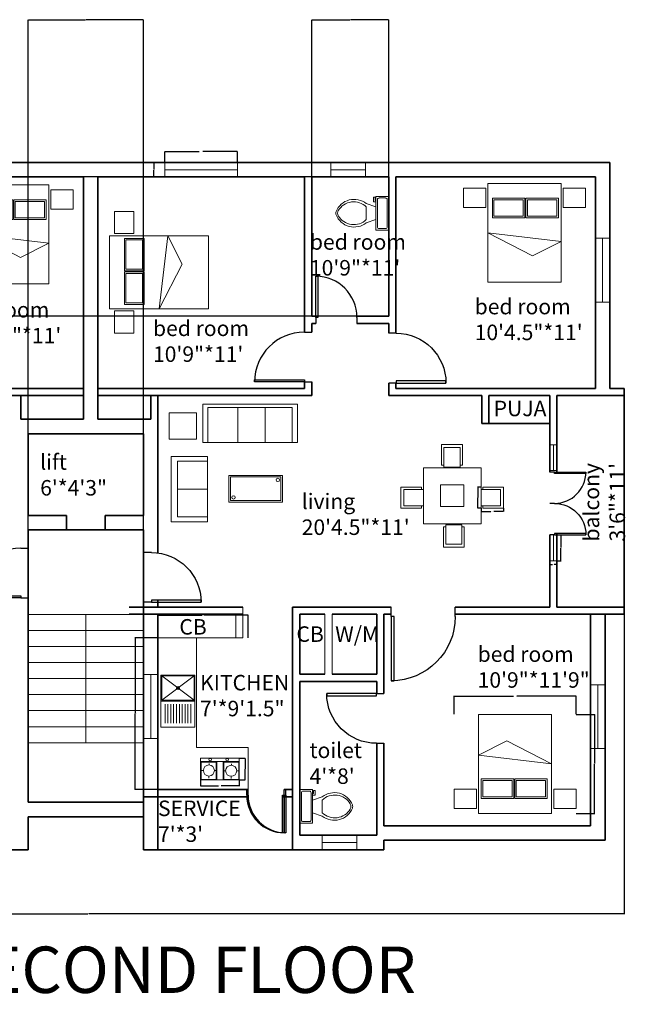
# Model space of a CAD drawing. Units: inches. Extents: x 1632 to 2336, y 1480 to 2095.
# Tile 2 of 2: x 1958 to 2336, y 1480 to 2095. Entities that reach past the tile are written whole.
import ezdxf

# ---------------------------------------------------------------- set-up
doc = ezdxf.new("R2010")
doc.units = ezdxf.units.IN
for name, color, linetype, lineweight in [('A-ANNO-DIMS', 2, 'Continuous', 18), ('A-ANNO-TEXT', 7, 'Continuous', 18), ('A-ANNO-TITL', 7, 'Continuous', 35), ('A-AREA-IDEN', 7, 'Continuous', 18), ('A-DOOR', 3, 'Continuous', 25), ('A-EQPM', 8, 'Continuous', 18), ('A-FLOR-CASE', 9, 'Continuous', 18), ('A-FLOR-FIXT', 9, 'Continuous', 18), ('A-FLOR-STRS', 7, 'Continuous', 18), ('A-FURN', 8, 'Continuous', 18), ('A-GLAZ', 4, 'Continuous', 18), ('A-WALL', 7, 'Continuous', 35)]:
    doc.layers.add(name, color=color, linetype=linetype, lineweight=lineweight)
doc.styles.get("Standard").update_dxf_attribs({"font": 'arial.ttf'})
doc.dimstyles.get("Standard").update_dxf_attribs({"dimtxt": 0.18, "dimasz": 0.18, "dimexe": 0.18, "dimexo": 0.0625, "dimgap": 0.09, "dimtad": 0, "dimtih": 1, "dimtoh": 1, "dimdec": 4, "dimzin": 0, "dimdsep": 46, "dimtxsty": 'Standard', "dimcen": 0.09, "dimadec": 0, "dimazin": 0, "dimtfac": 1, "dimtdec": 4, "dimtofl": 0, "dimtmove": 0, "dimatfit": 3, "dimfxl": 1, "dimtolj": 1, "dimtzin": 0, "dimarcsym": 0})

# ---------------------------------------------------------------- blocks, each defined once
blk = doc.blocks.new('*U2')
for p, q in [((0, 0), (0, -6)), ((40, 0), (40, -6))]:
    blk.add_line(p, q)
blk.add_lwpolyline([(0, 0), (0, 40), (1.75, 40), (1.75, 0)], close=True)
blk.add_arc((0, 0), 40, 0, 90)
blk = doc.blocks.new('*U4')
for p, q in [((9.5, -6), (9.5, -2)), ((-10, -8.5), (-8, -8.5)), ((-10, -9.5), (-10, -8.5)), ((-7, -9.5), (-10, -9.5)), ((-8, -8.5), (-8, -8)), ((-7, -8), (-7, -9.5)), ((-4, -8), (-6, -14)), ((4, -8), (6, -14)), ((4, -14), (-4, -14))]:
    blk.add_line(p, q)
blk.add_lwpolyline([(10.5, -8), (10.5, 0), (-10.5, 0), (-10.5, -8)], close=True)
for points in [[(-9.5, -2), (-9.5, -6)], [(8.5, -1), (-8.5, -1)], [(-8.5, -7), (8.5, -7)]]:
    blk.add_lwpolyline(points)
for centre, radius, start, end in [((-8.62, -1.88), 0.884, 81.8699, 188.1301), ((-8.62, -6.12), 0.884, 171.8699, 278.1301), ((8.62, -1.88), 0.884, 351.8699, 98.1301), ((8.62, -6.12), 0.884, 261.8699, 8.1301), ((3.52, -21.58), 12.17, 141.46911, 247.97143), ((4.2, -21.82), 11.33, 136.36773, 238.94682), ((-3.52, -21.58), 12.17, 292.02843, 38.53071), ((-4.2, -21.82), 11.33, 301.05301, 43.63209), ((0, -27.88), 4, 245.73182, 294.26817), ((0, -29), 4, 254.86053, 285.13947)]:
    blk.add_arc(centre, radius, start, end)
blk = doc.blocks.new('BED-DOUBLE-WITH-NIGHTSTANDS')
for p, q in [((30.9, 15.3), (36.28, 60.91)), ((36.28, 60.91), (45.27, 43.14)), ((45.27, 43.14), (30.9, 15.3))]:
    blk.add_line(p, q)
for points in [[(3.09, 62.18), (15.1, 62.18), (15.1, 76.08), (3.09, 76.08)], [(0, 15.3), (61.8, 15.3), (61.8, 60.91), (0, 60.91)], [(9.26, 38.94), (21.51, 38.94), (21.51, 59.23), (9.26, 59.23)], [(10.26, 39.94), (20.51, 39.94), (20.51, 58.23), (10.26, 58.23)], [(9.26, 18.02), (21.51, 18.02), (21.51, 38.31), (9.26, 38.31)], [(10.26, 19.02), (20.51, 19.02), (20.51, 37.31), (10.26, 37.31)], [(3.09, 0), (15.1, 0), (15.1, 13.9), (3.09, 13.9)]]:
    blk.add_lwpolyline(points, close=True)
blk = doc.blocks.new('CHAIR-DINING')
for p, q in [((0, 1.12), (0, 13.97)), ((0, 13.97), (12.95, 13.97)), ((12.95, 13.97), (12.95, 1.12)), ((1.47, 1.12), (0, 1.12)), ((12.95, 1.12), (11.55, 1.12))]:
    blk.add_line(p, q)
blk.add_lwpolyline([(1.47, 0), (11.55, 0), (11.55, 12.08), (1.47, 12.08)], close=True)
blk = doc.blocks.new('TABLE-DINING')
for points in [[(0, 35.03), (36, 35.03), (36, 0), (0, 0)], [(10.77, 24.25), (25.23, 24.25), (25.23, 10.77), (10.77, 10.77)]]:
    blk.add_lwpolyline(points, close=True)
blk = doc.blocks.new('SOFA-3-SEAT')
for p, q in [((0, 0), (0, 24.07)), ((0, 24.07), (59, 24.07)), ((20.13, 21.83), (20.13, 0)), ((37.25, 21.83), (37.25, 0)), ((59, 0), (59, 24.07)), ((3.41, 0), (0, 0)), ((56, 0), (59, 0))]:
    blk.add_line(p, q)
blk.add_lwpolyline([(3.41, 21.83), (56, 21.83), (56, 0), (3.41, 0)], close=True)
blk = doc.blocks.new('SOFA-2-SEAT')
for p, q in [((0, 37.84), (0, 40.84)), ((0, 40.84), (22.7, 40.84)), ((22.7, 40.84), (22.7, 0)), ((0, 20.42), (18.79, 20.42)), ((0, 3), (0, 0)), ((0, 0), (22.7, 0))]:
    blk.add_line(p, q)
blk.add_lwpolyline([(18.79, 37.84), (0, 37.84), (0, 3), (18.79, 3)], close=True)
blk = doc.blocks.new('TABLE-COFFEE')
for points in [[(0, 16.65), (33.49, 16.65), (33.49, 0), (0, 0)], [(1, 15.65), (32.49, 15.65), (32.49, 1), (1, 1)]]:
    blk.add_lwpolyline(points, close=True)
for centre in [(2.89, 13.8), (30.54, 2.86)]:
    blk.add_circle(centre, 1.06)
blk = doc.blocks.new('SINK-WITH-DRAINBOARD')
for p, q in [((0.63, 16.78), (20.68, 31.97)), ((0.63, 31.97), (20.68, 16.78)), ((0, 16.25), (21.16, 16.25)), ((2.61, 14.26), (2.61, 2.54)), ((4.39, 14.26), (4.39, 2.54)), ((6.16, 14.26), (6.16, 2.54)), ((7.94, 14.26), (7.94, 2.54)), ((9.72, 14.26), (9.72, 2.54)), ((11.49, 14.26), (11.49, 2.54)), ((13.27, 14.26), (13.27, 2.54)), ((15.04, 14.26), (15.04, 2.54)), ((16.82, 14.26), (16.82, 2.54)), ((18.6, 14.26), (18.6, 2.54))]:
    blk.add_line(p, q)
for points in [[(0, 0), (21.16, 0), (21.16, 32.49), (0, 32.49)], [(0.63, 31.97), (20.68, 31.97), (20.68, 16.78), (0.63, 16.78)]]:
    blk.add_lwpolyline(points, close=True)
blk.add_circle((10.66, 24.37), 0.977)
blk = doc.blocks.new('COOKTOP-2-BURNER')
for p, q in [((0, 11.46), (0, 13.65)), ((0, 13.65), (24.07, 13.65)), ((24.07, 13.65), (24.07, 11.46)), ((0, 11.46), (12, 11.46)), ((0, 11.46), (10, 11.46)), ((5.23, 9.36), (5.23, 10.33)), ((10, 11.46), (10, 0)), ((24.07, 11.46), (14.07, 11.46)), ((14.07, 11.46), (14.07, 0)), ((19.15, 9.18), (19.15, 10.15)), ((1.67, 5.97), (0.82, 5.97)), ((5.05, 2.47), (5.05, 1.13)), ((8.57, 5.88), (9.52, 5.88)), ((15.59, 5.79), (14.74, 5.79)), ((18.97, 2.28), (18.97, 0.95)), ((22.49, 5.7), (23.44, 5.7))]:
    blk.add_line(p, q)
for points in [[(0, 11.46), (24.07, 11.46), (24.07, 0), (0, 0)], [(0.38, 11.07), (9.77, 11.07), (9.77, 0.28), (0.38, 0.28)], [(14.37, 11.14), (23.83, 11.14), (23.83, 0.28), (14.37, 0.28)]]:
    blk.add_lwpolyline(points, close=True)
for centre, radius in [((5.93, 12.7), 0.782), ((16.53, 12.66), 0.782), ((5.12, 5.91), 3.45), ((19.04, 5.73), 3.45)]:
    blk.add_circle(centre, radius)
blk = doc.blocks.new('WINDOW-40')
blk.add_line((4.5, 39.93), (4.5, 0))
blk.add_lwpolyline([(0, 39.93), (9, 39.93), (9, 0), (0, 0)], close=True)
blk = doc.blocks.new('WINDOW-22')
blk.add_line((0, 4.5), (21.58, 4.5))
blk.add_lwpolyline([(0, 9), (21.58, 9), (21.58, 0), (0, 0)], close=True)
blk = doc.blocks.new('WINDOW-45')
blk.add_line((0, 4.5), (45.36, 4.5))
blk.add_lwpolyline([(0, 9), (45.36, 9), (45.36, 0), (0, 0)], close=True)
blk = doc.blocks.new('WINDOW-SIDELIGHT-16')
blk.add_line((2.25, 0), (2.25, 16.22))
blk.add_lwpolyline([(4.5, 0), (0, 0), (0, 16.22), (4.5, 16.22)], close=True)
blk = doc.blocks.new('TABLE-END')
blk.add_lwpolyline([(0, 16.51), (17.12, 16.51), (17.12, 0), (0, 0)], close=True)
blk = doc.blocks.new('COUNTERTOP-L-RETURN')
for p, q in [((0, 94.74), (24, 94.74)), ((24, 94.74), (24, 26.35)), ((24, 26.35), (56.24, 26.35)), ((56.24, 0), (56.24, 26.35))]:
    blk.add_line(p, q)
blk = doc.blocks.new('*D20')
at = {"layer": 'A-ANNO-DIMS', "color": 0, "lineweight": -2, "transparency": 16777216}
for p, q in [((2229, 1661.18), (2229, 1672.71)), ((2229.18, 1672.53), (2265.94, 1672.53)), ((2304.9, 1672.53), (2268.14, 1672.53)), ((2305.08, 1661.18), (2305.08, 1672.71))]:
    blk.add_line(p, q, dxfattribs=at)
at = {"layer": 'A-ANNO-DIMS', "color": 0, "transparency": 16777216}
for points in [[(2229.18, 1672.56), (2229.18, 1672.5), (2229, 1672.53)], [(2304.9, 1672.56), (2304.9, 1672.5), (2305.08, 1672.53)]]:
    blk.add_solid(points, dxfattribs=at)
at = {"layer": 'Defpoints', "color": 0, "transparency": 16777216}
for p in [(2229, 1672.53), (2229, 1661.12), (2305.08, 1661.12)]:
    blk.add_point(p, dxfattribs=at)
at = {"layer": 'A-ANNO-DIMS', "color": 0, "transparency": 16777216, "insert": (2267.04, 1672.53), "char_height": 0.18, "attachment_point": 5}
blk.add_mtext('\\A1;BED SET 76 TYP.', dxfattribs=at)
blk = doc.blocks.new('*D21')
at = {"layer": 'A-ANNO-DIMS', "color": 0, "lineweight": -2, "transparency": 16777216}
for p, q in [((2305.14, 1661.12), (2316.67, 1661.12)), ((2316.49, 1660.94), (2316.49, 1630.4)), ((2316.49, 1599.5), (2316.49, 1630.04)), ((2305.14, 1599.32), (2316.67, 1599.32))]:
    blk.add_line(p, q, dxfattribs=at)
at = {"layer": 'A-ANNO-DIMS', "color": 0, "transparency": 16777216}
for points in [[(2316.46, 1660.94), (2316.52, 1660.94), (2316.49, 1661.12)], [(2316.46, 1599.5), (2316.52, 1599.5), (2316.49, 1599.32)]]:
    blk.add_solid(points, dxfattribs=at)
at = {"layer": 'Defpoints', "color": 0, "transparency": 16777216}
for p in [(2305.08, 1661.12), (2316.49, 1661.12), (2305.08, 1599.32)]:
    blk.add_point(p, dxfattribs=at)
at = {"layer": 'A-ANNO-DIMS', "color": 0, "transparency": 16777216, "insert": (2316.49, 1630.22), "char_height": 0.18, "attachment_point": 5}
blk.add_mtext('\\A1;62 TYP.', dxfattribs=at)
blk = doc.blocks.new('*D22')
at = {"layer": 'A-ANNO-DIMS', "color": 0, "lineweight": -2, "transparency": 16777216}
for p, q in [((2245.75, 1789.88), (2245.75, 1787.66)), ((2259.72, 1789.88), (2259.72, 1787.66)), ((2245.93, 1787.84), (2251.78, 1787.84)), ((2259.54, 1787.84), (2253.69, 1787.84))]:
    blk.add_line(p, q, dxfattribs=at)
at = {"layer": 'A-ANNO-DIMS', "color": 0, "transparency": 16777216}
for points in [[(2245.93, 1787.87), (2245.93, 1787.81), (2245.75, 1787.84)], [(2259.54, 1787.87), (2259.54, 1787.81), (2259.72, 1787.84)]]:
    blk.add_solid(points, dxfattribs=at)
at = {"layer": 'Defpoints', "color": 0, "transparency": 16777216}
for p in [(2245.75, 1789.94), (2259.72, 1789.94), (2259.72, 1787.84)]:
    blk.add_point(p, dxfattribs=at)
at = {"layer": 'A-ANNO-DIMS', "color": 0, "transparency": 16777216, "insert": (2252.74, 1787.84), "char_height": 0.18, "attachment_point": 5}
blk.add_mtext('\\A1;CHAIR 14 TYP.', dxfattribs=at)
blk = doc.blocks.new('*D23')
at = {"layer": 'A-ANNO-DIMS', "color": 0, "lineweight": -2, "transparency": 16777216}
for p, q in [((2245.69, 1802.89), (2243.48, 1802.89)), ((2243.66, 1802.71), (2243.66, 1796.6)), ((2243.66, 1790.12), (2243.66, 1796.23)), ((2245.69, 1789.94), (2243.48, 1789.94))]:
    blk.add_line(p, q, dxfattribs=at)
at = {"layer": 'A-ANNO-DIMS', "color": 0, "transparency": 16777216}
for points in [[(2243.63, 1802.71), (2243.69, 1802.71), (2243.66, 1802.89)], [(2243.63, 1790.12), (2243.69, 1790.12), (2243.66, 1789.94)]]:
    blk.add_solid(points, dxfattribs=at)
at = {"layer": 'Defpoints', "color": 0, "transparency": 16777216}
for p in [(2245.75, 1802.89), (2243.66, 1789.94), (2245.75, 1789.94)]:
    blk.add_point(p, dxfattribs=at)
at = {"layer": 'A-ANNO-DIMS', "color": 0, "transparency": 16777216, "insert": (2243.66, 1796.41), "char_height": 0.18, "attachment_point": 5}
blk.add_mtext('\\A1;13 TYP.', dxfattribs=at)
blk = doc.blocks.new('*D38')
at = {"layer": 'A-ANNO-DIMS', "color": 0, "lineweight": -2, "transparency": 16777216}
for p, q in [((2048.38, 2005.69), (2048.38, 2012.61)), ((2048.56, 2012.43), (2069.94, 2012.43)), ((2093.56, 2012.43), (2072.18, 2012.43)), ((2093.74, 2005.69), (2093.74, 2012.61))]:
    blk.add_line(p, q, dxfattribs=at)
at = {"layer": 'A-ANNO-DIMS', "color": 0, "transparency": 16777216}
for points in [[(2048.56, 2012.46), (2048.56, 2012.4), (2048.38, 2012.43)], [(2093.56, 2012.46), (2093.56, 2012.4), (2093.74, 2012.43)]]:
    blk.add_solid(points, dxfattribs=at)
at = {"layer": 'Defpoints', "color": 0, "transparency": 16777216}
for p in [(2093.74, 2012.43), (2048.38, 2005.62), (2093.74, 2005.62)]:
    blk.add_point(p, dxfattribs=at)
at = {"layer": 'A-ANNO-DIMS', "color": 0, "transparency": 16777216, "insert": (2071.06, 2012.43), "char_height": 0.18, "attachment_point": 5}
blk.add_mtext('\\A1;WINDOW 45 TYP.', dxfattribs=at)
blk = doc.blocks.new('*D39')
at = {"layer": 'A-ANNO-DIMS', "color": 0, "lineweight": -2, "transparency": 16777216}
for p, q in [((2048.32, 2005.62), (2041.4, 2005.62)), ((2041.58, 2005.44), (2041.58, 2001.31)), ((2041.58, 1996.8), (2041.58, 2000.94)), ((2048.32, 1996.62), (2041.4, 1996.62))]:
    blk.add_line(p, q, dxfattribs=at)
at = {"layer": 'A-ANNO-DIMS', "color": 0, "transparency": 16777216}
for points in [[(2041.55, 2005.44), (2041.61, 2005.44), (2041.58, 2005.62)], [(2041.55, 1996.8), (2041.61, 1996.8), (2041.58, 1996.62)]]:
    blk.add_solid(points, dxfattribs=at)
at = {"layer": 'Defpoints', "color": 0, "transparency": 16777216}
for p in [(2041.58, 2005.62), (2048.38, 2005.62), (2048.38, 1996.62)]:
    blk.add_point(p, dxfattribs=at)
at = {"layer": 'A-ANNO-DIMS', "color": 0, "transparency": 16777216, "insert": (2041.58, 2001.12), "char_height": 0.18, "attachment_point": 5}
blk.add_mtext('\\A1;9 TYP.', dxfattribs=at)
blk = doc.blocks.new('*D40')
at = {"layer": 'A-ANNO-DIMS', "color": 0, "lineweight": -2, "transparency": 16777216}
for p, q in [((2293.21, 1773.25), (2295.76, 1773.25)), ((2295.58, 1773.07), (2295.58, 1765.32)), ((2295.58, 1757.21), (2295.58, 1764.96)), ((2293.21, 1757.03), (2295.76, 1757.03))]:
    blk.add_line(p, q, dxfattribs=at)
at = {"layer": 'A-ANNO-DIMS', "color": 0, "transparency": 16777216}
for points in [[(2295.55, 1773.07), (2295.61, 1773.07), (2295.58, 1773.25)], [(2295.55, 1757.21), (2295.61, 1757.21), (2295.58, 1757.03)]]:
    blk.add_solid(points, dxfattribs=at)
at = {"layer": 'Defpoints', "color": 0, "transparency": 16777216}
for p in [(2293.15, 1773.25), (2295.58, 1773.25), (2293.15, 1757.03)]:
    blk.add_point(p, dxfattribs=at)
at = {"layer": 'A-ANNO-DIMS', "color": 0, "transparency": 16777216, "insert": (2295.58, 1765.14), "char_height": 0.18, "attachment_point": 5}
blk.add_mtext('\\A1;SIDELIGHT 16 TYP.', dxfattribs=at)
blk = doc.blocks.new('*D41')
at = {"layer": 'A-ANNO-DIMS', "color": 0, "lineweight": -2, "transparency": 16777216}
for p, q in [((2288.65, 1756.97), (2288.65, 1754.42)), ((2288.83, 1754.6), (2290.44, 1754.6)), ((2292.97, 1754.6), (2291.36, 1754.6)), ((2293.15, 1756.97), (2293.15, 1754.42))]:
    blk.add_line(p, q, dxfattribs=at)
at = {"layer": 'A-ANNO-DIMS', "color": 0, "transparency": 16777216}
for points in [[(2288.83, 1754.63), (2288.83, 1754.57), (2288.65, 1754.6)], [(2292.97, 1754.63), (2292.97, 1754.57), (2293.15, 1754.6)]]:
    blk.add_solid(points, dxfattribs=at)
at = {"layer": 'Defpoints', "color": 0, "transparency": 16777216}
for p in [(2288.65, 1757.03), (2293.15, 1757.03), (2293.15, 1754.6)]:
    blk.add_point(p, dxfattribs=at)
at = {"layer": 'A-ANNO-DIMS', "color": 0, "transparency": 16777216, "insert": (2290.9, 1754.6), "char_height": 0.18, "attachment_point": 5}
blk.add_mtext('\\A1;5 TYP.', dxfattribs=at)
blk = doc.blocks.new('*D44')
at = {"layer": 'A-ANNO-DIMS', "color": 0, "lineweight": -2, "transparency": 16777216}
for p, q in [((2070.78, 1620.1), (2070.78, 1616.37)), ((2094.86, 1620.1), (2094.86, 1616.37)), ((2070.96, 1616.55), (2081.99, 1616.55)), ((2094.68, 1616.55), (2083.65, 1616.55))]:
    blk.add_line(p, q, dxfattribs=at)
at = {"layer": 'A-ANNO-DIMS', "color": 0, "transparency": 16777216}
for points in [[(2070.96, 1616.58), (2070.96, 1616.52), (2070.78, 1616.55)], [(2094.68, 1616.58), (2094.68, 1616.52), (2094.86, 1616.55)]]:
    blk.add_solid(points, dxfattribs=at)
at = {"layer": 'Defpoints', "color": 0, "transparency": 16777216}
for p in [(2070.78, 1620.16), (2094.86, 1620.16), (2094.86, 1616.55)]:
    blk.add_point(p, dxfattribs=at)
at = {"layer": 'A-ANNO-DIMS', "color": 0, "transparency": 16777216, "insert": (2082.82, 1616.55), "char_height": 0.18, "attachment_point": 5}
blk.add_mtext('\\A1;HOB 24 TYP.', dxfattribs=at)
blk = doc.blocks.new('*D45')
at = {"layer": 'A-ANNO-DIMS', "color": 0, "lineweight": -2, "transparency": 16777216}
for p, q in [((2094.92, 1633.81), (2098.65, 1633.81)), ((2098.47, 1633.63), (2098.47, 1627.17)), ((2098.47, 1620.34), (2098.47, 1626.81)), ((2094.92, 1620.16), (2098.65, 1620.16))]:
    blk.add_line(p, q, dxfattribs=at)
at = {"layer": 'A-ANNO-DIMS', "color": 0, "transparency": 16777216}
for points in [[(2098.44, 1633.63), (2098.5, 1633.63), (2098.47, 1633.81)], [(2098.44, 1620.34), (2098.5, 1620.34), (2098.47, 1620.16)]]:
    blk.add_solid(points, dxfattribs=at)
at = {"layer": 'Defpoints', "color": 0, "transparency": 16777216}
for p in [(2094.86, 1633.81), (2098.47, 1633.81), (2094.86, 1620.16)]:
    blk.add_point(p, dxfattribs=at)
at = {"layer": 'A-ANNO-DIMS', "color": 0, "transparency": 16777216, "insert": (2098.47, 1626.99), "char_height": 0.18, "attachment_point": 5}
blk.add_mtext('\\A1;14 TYP.', dxfattribs=at)
blk = doc.blocks.new('*D46')
at = {"layer": 'A-ANNO-DIMS', "color": 0, "lineweight": -2, "transparency": 16777216}
for p, q in [((2044.09, 1708.87), (2029.76, 1708.87)), ((2029.94, 1708.69), (2029.94, 1661.68)), ((2029.94, 1614.3), (2029.94, 1661.31)), ((2044.09, 1614.12), (2029.76, 1614.12))]:
    blk.add_line(p, q, dxfattribs=at)
at = {"layer": 'A-ANNO-DIMS', "color": 0, "transparency": 16777216}
for points in [[(2029.91, 1708.69), (2029.97, 1708.69), (2029.94, 1708.87)], [(2029.91, 1614.3), (2029.97, 1614.3), (2029.94, 1614.12)]]:
    blk.add_solid(points, dxfattribs=at)
at = {"layer": 'Defpoints', "color": 0, "transparency": 16777216}
for p in [(2029.94, 1708.87), (2044.15, 1708.87), (2044.15, 1614.12)]:
    blk.add_point(p, dxfattribs=at)
at = {"layer": 'A-ANNO-DIMS', "color": 0, "transparency": 16777216, "insert": (2029.94, 1661.5), "char_height": 0.18, "attachment_point": 5}
blk.add_mtext('\\A1;COUNTER 95 TYP.', dxfattribs=at)
blk = doc.blocks.new('*D47')
at = {"layer": 'A-ANNO-DIMS', "color": 0, "lineweight": -2, "transparency": 16777216}
for p, q in [((2044.15, 1708.93), (2044.15, 1723.26)), ((2044.33, 1723.08), (2071.74, 1723.08)), ((2100.21, 1723.08), (2072.8, 1723.08)), ((2100.39, 1708.93), (2100.39, 1723.26))]:
    blk.add_line(p, q, dxfattribs=at)
at = {"layer": 'A-ANNO-DIMS', "color": 0, "transparency": 16777216}
for points in [[(2044.33, 1723.11), (2044.33, 1723.05), (2044.15, 1723.08)], [(2100.21, 1723.11), (2100.21, 1723.05), (2100.39, 1723.08)]]:
    blk.add_solid(points, dxfattribs=at)
at = {"layer": 'Defpoints', "color": 0, "transparency": 16777216}
for p in [(2100.39, 1723.08), (2044.15, 1708.87), (2100.39, 1708.87)]:
    blk.add_point(p, dxfattribs=at)
at = {"layer": 'A-ANNO-DIMS', "color": 0, "transparency": 16777216, "insert": (2072.27, 1723.08), "char_height": 0.18, "attachment_point": 5}
blk.add_mtext('\\A1;56 TYP.', dxfattribs=at)
blk = doc.blocks.new('*D48')
at = {"layer": 'A-ANNO-DIMS', "color": 0, "lineweight": -2, "transparency": 16777216}
for p, q in [((1666.2, 1731.06), (1666.2, 1536.39)), ((2335.15, 1728.06), (2335.15, 1536.39)), ((1666.38, 1536.57), (2000.39, 1536.57)), ((2334.97, 1536.57), (2000.97, 1536.57))]:
    blk.add_line(p, q, dxfattribs=at)
at = {"layer": 'A-ANNO-DIMS', "color": 0, "transparency": 16777216}
for points in [[(1666.38, 1536.6), (1666.38, 1536.54), (1666.2, 1536.57)], [(2334.97, 1536.6), (2334.97, 1536.54), (2335.15, 1536.57)]]:
    blk.add_solid(points, dxfattribs=at)
at = {"layer": 'Defpoints', "color": 0, "transparency": 16777216}
for p in [(1666.2, 1731.12), (2335.15, 1728.12), (2335.15, 1536.57)]:
    blk.add_point(p, dxfattribs=at)
at = {"layer": 'A-ANNO-DIMS', "color": 0, "transparency": 16777216, "insert": (2000.68, 1536.57), "char_height": 0.18, "attachment_point": 5}
blk.add_mtext('\\A1;669', dxfattribs=at)
blk = doc.blocks.new('*D50')
at = {"layer": 'A-ANNO-DIMS', "color": 0, "lineweight": -2, "transparency": 16777216}
for p, q in [((1963.15, 1723.48), (1963.15, 2094.81)), ((1963.33, 2094.63), (1998.93, 2094.63)), ((2034.97, 2094.63), (1999.37, 2094.63)), ((2035.15, 1723.69), (2035.15, 2094.81))]:
    blk.add_line(p, q, dxfattribs=at)
at = {"layer": 'A-ANNO-DIMS', "color": 0, "transparency": 16777216}
for points in [[(1963.33, 2094.66), (1963.33, 2094.6), (1963.15, 2094.63)], [(2034.97, 2094.66), (2034.97, 2094.6), (2035.15, 2094.63)]]:
    blk.add_solid(points, dxfattribs=at)
at = {"layer": 'Defpoints', "color": 0, "transparency": 16777216}
for p in [(2035.15, 2094.63), (1963.15, 1723.42), (2035.15, 1723.62)]:
    blk.add_point(p, dxfattribs=at)
at = {"layer": 'A-ANNO-DIMS', "color": 0, "transparency": 16777216, "insert": (1999.15, 2094.63), "char_height": 0.18, "attachment_point": 5}
blk.add_mtext('\\A1;72', dxfattribs=at)
blk = doc.blocks.new('*D51')
at = {"layer": 'A-ANNO-DIMS', "color": 0, "lineweight": -2, "transparency": 16777216}
for p, q in [((2140.15, 1996.69), (2140.15, 2094.81)), ((2140.33, 2094.63), (2163.93, 2094.63)), ((2187.97, 2094.63), (2164.37, 2094.63)), ((2188.15, 1996.69), (2188.15, 2094.81))]:
    blk.add_line(p, q, dxfattribs=at)
at = {"layer": 'A-ANNO-DIMS', "color": 0, "transparency": 16777216}
for points in [[(2140.33, 2094.66), (2140.33, 2094.6), (2140.15, 2094.63)], [(2187.97, 2094.66), (2187.97, 2094.6), (2188.15, 2094.63)]]:
    blk.add_solid(points, dxfattribs=at)
at = {"layer": 'Defpoints', "color": 0, "transparency": 16777216}
for p in [(2188.15, 2094.63), (2140.15, 1996.62), (2188.15, 1996.62)]:
    blk.add_point(p, dxfattribs=at)
at = {"layer": 'A-ANNO-DIMS', "color": 0, "transparency": 16777216, "insert": (2164.15, 2094.63), "char_height": 0.18, "attachment_point": 5}
blk.add_mtext('\\A1;48', dxfattribs=at)
blk = doc.blocks.new('*D52')
at = {"layer": 'A-ANNO-DIMS', "color": 0, "lineweight": -2, "transparency": 16777216}
for p, q in [((2188.09, 1996.62), (1631.97, 1996.62)), ((1632.15, 1996.44), (1632.15, 1953.31)), ((1632.15, 1909.8), (1632.15, 1952.94)), ((2188.09, 1909.62), (1631.97, 1909.62))]:
    blk.add_line(p, q, dxfattribs=at)
at = {"layer": 'A-ANNO-DIMS', "color": 0, "transparency": 16777216}
for points in [[(1632.12, 1996.44), (1632.18, 1996.44), (1632.15, 1996.62)], [(1632.12, 1909.8), (1632.18, 1909.8), (1632.15, 1909.62)]]:
    blk.add_solid(points, dxfattribs=at)
at = {"layer": 'Defpoints', "color": 0, "transparency": 16777216}
for p in [(1632.15, 1996.62), (2188.15, 1996.62), (2188.15, 1909.62)]:
    blk.add_point(p, dxfattribs=at)
at = {"layer": 'A-ANNO-DIMS', "color": 0, "transparency": 16777216, "insert": (1632.15, 1953.12), "char_height": 0.18, "attachment_point": 5}
blk.add_mtext('\\A1;87', dxfattribs=at)

msp = doc.modelspace()

# ---------------------------------------------------------------- linework, layer by layer
at = {"layer": 'A-FLOR-CASE'}
for p, q in [((2097.15, 1728.12), (2097.15, 1708.87)), ((2092.65, 1723.62), (2092.65, 1708.87)), ((2148.27, 1723.62), (2148.27, 1686.12)), ((2152.77, 1723.62), (2152.77, 1686.12)), ((2097.15, 1708.87), (2044.15, 1708.87))]:
    msp.add_line(p, q, dxfattribs=at)
at = {"layer": 'A-FLOR-STRS'}
for p, q in [((1963.15, 1723.42), (2035.15, 1723.42)), ((1999.15, 1723.42), (1999.15, 1648.81)), ((1963.15, 1713.42), (2035.15, 1713.42)), ((1963.15, 1703.42), (2035.15, 1703.42)), ((1963.15, 1693.42), (2035.15, 1693.42)), ((1963.15, 1683.42), (2035.15, 1683.42)), ((1963.15, 1673.42), (2035.15, 1673.42)), ((1963.15, 1663.42), (2035.15, 1663.42)), ((1963.15, 1653.42), (2035.15, 1653.42)), ((1999.15, 1648.81), (1999.15, 1643.42)), ((1963.15, 1643.42), (2035.15, 1643.42))]:
    msp.add_line(p, q, dxfattribs=at)
at = {"layer": 'A-WALL'}
for p, q in [((1873.15, 2005.62), (2006.65, 2005.62)), ((2006.65, 2005.62), (2140.15, 2005.62)), ((2140.15, 2005.62), (2192.65, 2005.62)), ((2192.65, 2005.62), (2326.15, 2005.62)), ((2326.15, 2005.62), (2326.15, 1864.62)), ((1873.15, 1996.62), (1997.65, 1996.62)), ((1997.65, 1996.62), (1997.65, 1864.62)), ((2006.65, 1996.62), (2006.65, 1864.62)), ((2006.65, 1996.62), (2135.65, 1996.62)), ((2135.65, 1996.62), (2135.65, 1899.72)), ((2140.15, 1996.62), (2140.15, 1909.62)), ((2140.15, 1996.62), (2188.15, 1996.62)), ((2188.15, 1996.62), (2188.15, 1909.62)), ((2192.65, 1996.62), (2192.65, 1905.12)), ((2192.65, 1996.62), (2317.15, 1996.62)), ((2317.15, 1996.62), (2317.15, 1864.62)), ((2143.8, 1909.62), (2140.15, 1909.62)), ((2188.15, 1909.62), (2168.31, 1909.62)), ((2140.15, 1905.12), (2140.15, 1899.72)), ((2142.68, 1905.12), (2140.15, 1905.12)), ((2188.15, 1905.12), (2168.32, 1905.12)), ((2188.15, 1899.01), (2188.15, 1905.12)), ((2192.65, 1899.01), (2192.65, 1905.12)), ((1997.65, 1864.62), (1873.15, 1864.62)), ((1997.65, 1864.62), (1997.65, 1845.35)), ((2135.65, 1864.62), (2006.65, 1864.62)), ((2006.65, 1864.62), (2006.65, 1845.35)), ((2135.65, 1868.66), (2135.65, 1864.62)), ((2140.15, 1868.66), (2140.15, 1860.12)), ((2188.15, 1860.12), (2188.15, 1867.95)), ((2192.65, 1864.62), (2192.65, 1867.95)), ((2317.15, 1864.62), (2192.65, 1864.62)), ((2326.15, 1864.62), (2335.15, 1864.62)), ((2335.15, 1864.62), (2335.15, 1723.62)), ((1997.65, 1860.12), (1868.65, 1860.12)), ((1958.65, 1845.35), (1958.65, 1860.12)), ((2035.15, 1860.12), (2006.65, 1860.12)), ((2140.15, 1860.12), (2006.65, 1860.12)), ((2039.65, 1860.12), (2039.65, 1845.35)), ((2044.15, 1845.35), (2044.15, 1860.12)), ((2044.15, 1860.12), (2044.15, 1761.88)), ((2246.15, 1860.12), (2188.15, 1860.12)), ((2246.15, 1860.12), (2246.15, 1842.62)), ((2252.65, 1860.12), (2250.65, 1860.12)), ((2250.65, 1860.12), (2250.65, 1842.62)), ((2288.65, 1860.12), (2250.65, 1860.12)), ((2288.65, 1860.12), (2252.65, 1860.12)), ((2288.65, 1812.4), (2288.65, 1860.12)), ((2326.15, 1860.12), (2293.15, 1860.12)), ((2293.15, 1860.12), (2335.15, 1860.12)), ((2293.15, 1811.55), (2293.15, 1860.12)), ((1958.65, 1845.35), (1997.65, 1845.35)), ((2006.65, 1845.35), (2039.65, 1845.35)), ((2044.15, 1776.35), (2044.15, 1845.35)), ((2246.15, 1842.62), (2288.65, 1842.62)), ((1963.15, 1836.35), (1963.15, 1785.35)), ((1963.15, 1836.35), (2035.15, 1836.35)), ((2035.15, 1785.35), (2035.15, 1836.35)), ((1963.15, 1785.35), (1963.15, 1822.53)), ((1963.15, 1785.35), (1963.15, 1788.98)), ((2293.15, 1792.76), (2293.15, 1792.89)), ((1963.15, 1785.35), (1987.15, 1785.35)), ((1987.15, 1776.35), (1987.15, 1785.35)), ((2011.15, 1776.35), (2011.15, 1785.35)), ((2011.15, 1785.35), (2035.15, 1785.35)), ((1963.15, 1719.98), (1963.15, 1776.35)), ((1963.15, 1776.35), (2035.15, 1776.35)), ((1963.15, 1776.35), (1987.15, 1776.35)), ((2035.15, 1776.35), (2011.15, 1776.35)), ((2035.15, 1776.35), (2035.15, 1606.23)), ((2288.65, 1728.12), (2288.65, 1773.25)), ((2293.15, 1728.12), (2293.15, 1774.1)), ((1963.15, 1606.23), (1963.15, 1731.12)), ((2068.2, 1728.12), (2026.2, 1728.12)), ((2044.15, 1732.45), (2044.15, 1728.12)), ((2044.15, 1728.12), (2097.15, 1728.12)), ((2097.15, 1728.12), (2072.7, 1728.12)), ((2128.15, 1723.62), (2128.15, 1728.12)), ((2128.15, 1728.12), (2189.69, 1728.12)), ((2229.69, 1728.12), (2288.65, 1728.12)), ((2335.15, 1728.12), (2293.15, 1728.12)), ((2072.7, 1723.62), (2026.2, 1723.62)), ((2035.15, 1723.62), (2035.15, 1609.62)), ((2044.15, 1723.62), (2097.15, 1723.62)), ((2044.15, 1723.62), (2044.15, 1585.62)), ((2044.15, 1723.62), (2097.15, 1723.62)), ((2044.15, 1723.62), (2044.15, 1614.12)), ((2092.65, 1723.62), (2072.7, 1723.62)), ((2128.15, 1723.62), (2128.15, 1614.12)), ((2128.15, 1614.12), (2128.15, 1723.62)), ((2132.65, 1723.62), (2132.65, 1686.12)), ((2132.65, 1723.62), (2148.27, 1723.62)), ((2152.77, 1723.62), (2180.65, 1723.62)), ((2180.65, 1686.12), (2180.65, 1723.62)), ((2185.15, 1686.12), (2185.15, 1723.62)), ((2185.15, 1723.62), (2189.69, 1723.62)), ((2185.15, 1723.62), (2189.69, 1723.62)), ((2229.69, 1723.62), (2314.15, 1723.62)), ((2229.69, 1723.62), (2293.15, 1723.62)), ((2335.15, 1723.62), (2293.15, 1723.62)), ((2314.15, 1723.62), (2314.15, 1591.62)), ((2323.15, 1723.62), (2323.15, 1582.62)), ((2128.15, 1585.62), (2128.15, 1695.12)), ((2132.65, 1686.12), (2132.65, 1695.12)), ((2148.27, 1686.12), (2132.65, 1686.12)), ((2180.65, 1686.12), (2152.77, 1686.12)), ((2185.15, 1674.1), (2185.15, 1686.12)), ((2132.65, 1585.62), (2132.65, 1681.62)), ((2180.65, 1681.62), (2132.65, 1681.62)), ((2132.65, 1681.62), (2132.65, 1614.12)), ((2180.65, 1674.1), (2180.65, 1681.62)), ((2180.65, 1585.62), (2180.65, 1643.03)), ((2185.15, 1591.62), (2185.15, 1643.03)), ((2044.15, 1609.62), (2044.15, 1628.26)), ((2099.53, 1614.12), (2044.15, 1614.12)), ((2044.15, 1614.12), (2100.39, 1614.12)), ((2128.15, 1614.12), (2122.97, 1614.12)), ((2123.84, 1614.12), (2128.15, 1614.12)), ((2035.15, 1606.23), (1963.15, 1606.23)), ((2035.15, 1609.62), (2100.42, 1609.62)), ((2035.15, 1609.62), (2035.15, 1576.62)), ((2099.55, 1609.62), (2044.15, 1609.62)), ((2044.15, 1609.62), (2044.15, 1576.62)), ((2128.15, 1609.62), (2121.95, 1609.62)), ((2122.81, 1609.62), (2128.15, 1609.62)), ((2128.15, 1576.62), (2128.15, 1609.62)), ((1963.15, 1576.62), (1963.15, 1597.23)), ((2035.15, 1597.23), (1963.15, 1597.23)), ((2035.15, 1597.23), (2035.15, 1576.62)), ((2314.15, 1591.62), (2185.15, 1591.62)), ((2044.15, 1585.62), (2044.15, 1576.62)), ((2128.15, 1585.62), (2128.15, 1576.62)), ((2132.65, 1585.62), (2180.65, 1585.62)), ((2185.15, 1576.62), (2185.15, 1582.62)), ((2323.15, 1582.62), (2185.15, 1582.62)), ((1825.15, 1576.62), (1963.15, 1576.62)), ((2035.15, 1576.62), (2132.65, 1576.62)), ((2132.65, 1576.62), (2185.15, 1576.62))]:
    msp.add_line(p, q, dxfattribs=at)

# ---------------------------------------------------------------- block references
at = {"layer": 'A-DOOR', "xscale": 0.6408249326853631, "yscale": 0.6408249326853631, "zscale": 0.6408249326853631}
msp.add_blockref('*U2', (2142.68, 1908.97), dxfattribs=at)
at = {"layer": 'A-DOOR'}
for p, xscale, yscale, zscale, rotation in [((2135.49, 1868.66), 0.7765731612885453, 0.7765731612885453, 0.7765731612885453, 90), ((2192.81, 1867.95), -0.7765731612885453, 0.7765731612885453, 0.7765731612885453, 270), ((2291.59, 1812.4), 0.4894447198564081, 0.4894447198564081, 0.4894447198564081, 270), ((2291.59, 1773.25), -0.4894447198564081, 0.4894447198564081, 0.4894447198564081, 270), ((1958.49, 1733.78), 0.7765731612885453, 0.7765731612885453, 0.7765731612885453, 90), ((2040.02, 1731.09), -0.7765731612885453, 0.7765731612885453, 0.7765731612885453, 270), ((2180.49, 1674.1), -0.7765731612885453, 0.7765731612885453, 0.7765731612885453, 90), ((2122.97, 1610.61), 0.5860402873761541, 0.5860402873761541, 0.5860402873761541, 180), ((2123.84, 1610.61), 0.5860402873761541, 0.5860402873761541, 0.5860402873761541, 180)]:
    msp.add_blockref('*U2', p, dxfattribs=dict(at, xscale=xscale, yscale=yscale, zscale=zscale, rotation=rotation))
at = {"layer": 'A-DOOR', "xscale": -1, "rotation": 180}
msp.add_blockref('*U2', (2189.69, 1722.12), dxfattribs=at)
at = {"layer": 'A-EQPM'}
msp.add_blockref('COOKTOP-2-BURNER', (2070.78, 1620.16), dxfattribs=at)
at = {"layer": 'A-FLOR-CASE'}
msp.add_blockref('COUNTERTOP-L-RETURN', (2044.15, 1614.12), dxfattribs=at)
at = {"layer": 'A-FLOR-FIXT', "rotation": 270}
msp.add_blockref('*U4', (2188.15, 1973.99), dxfattribs=at)
at = {"layer": 'A-FLOR-FIXT'}
msp.add_blockref('SINK-WITH-DRAINBOARD', (2045.98, 1653.17), dxfattribs=at)
at = {"layer": 'A-FLOR-FIXT', "xscale": -1, "rotation": 90}
msp.add_blockref('*U4', (2132.65, 1603.62), dxfattribs=at)
at = {"layer": 'A-FURN'}
for name, p, rotation in [('BED-DOUBLE-WITH-NIGHTSTANDS', (2234.8, 1992.64), 270.0000000000004), ('BED-DOUBLE-WITH-NIGHTSTANDS', (1915.16, 1991.66), 269.9999999999999), ('CHAIR-DINING', (2245.75, 1802.89), 269.9999999999968), ('BED-DOUBLE-WITH-NIGHTSTANDS', (2305.08, 1599.32), 89.99999999999952)]:
    msp.add_blockref(name, p, dxfattribs=dict(at, rotation=rotation))
for name, p in [('BED-DOUBLE-WITH-NIGHTSTANDS', (2013.91, 1899.05)), ('CHAIR-DINING', (2221.15, 1815.54)), ('TABLE-DINING', (2209.75, 1780.06))]:
    msp.add_blockref(name, p, dxfattribs=at)
at = {"layer": 'A-FURN', "extrusion": (0, 0, -1), "zscale": -1}
for name, p in [('SOFA-3-SEAT', (-2131.19, 1830.78)), ('TABLE-END', (-2068.25, 1832.95)), ('SOFA-2-SEAT', (-2075.05, 1781.33)), ('TABLE-COFFEE', (-2121.81, 1793.67))]:
    msp.add_blockref(name, p, dxfattribs=at)
for p, rotation in [((-2209.75, 1802.89), 270), ((-2222.26, 1779.39), 180)]:
    msp.add_blockref('CHAIR-DINING', p, dxfattribs=dict(at, rotation=rotation))
at = {"layer": 'A-GLAZ'}
for name, p in [('WINDOW-45', (2048.38, 1996.62)), ('WINDOW-22', (2152.11, 1996.62)), ('WINDOW-40', (2317.15, 1918.39)), ('WINDOW-SIDELIGHT-16', (2288.65, 1813.26)), ('WINDOW-SIDELIGHT-16', (2288.65, 1757.03)), ('WINDOW-40', (2035.15, 1645.99)), ('WINDOW-40', (2314.15, 1639.7)), ('WINDOW-22', (2146.66, 1576.62))]:
    msp.add_blockref(name, p, dxfattribs=at)

# ---------------------------------------------------------------- texts
at = {"layer": 'A-ANNO-TEXT', "char_height": 9.673, "attachment_point": 1}
for s, insert in [('CB', (2057.47, 1720.59)), ('CB', (2130.55, 1716.05)), ('W/M', (2154.72, 1716.05))]:
    msp.add_mtext_dynamic_manual_height_columns(s, width=166.6207, gutter_width=48.36, heights=[0], dxfattribs=dict(at, insert=insert))
at = {"layer": 'A-ANNO-TITL', "insert": (1790.83, 1516.15), "char_height": 28.9764, "attachment_point": 1}
msp.add_mtext_dynamic_manual_height_columns('FIRST/SECOND FLOOR', width=499.1431, gutter_width=144.88, heights=[77.88], dxfattribs=at)
at = {"layer": 'A-AREA-IDEN', "attachment_point": 1}
for s, insert, char_height in [('bed room\\P10\'9"*11\'', (2138.95, 1960.88), 9.673), ('bed room\\P10\'4.5"*11\'', (1916.4, 1918.54), 9.6727), ('bed room\\P10\'4.5"*11\'', (2241.78, 1920.55), 9.6727), ('bed room\\P10\'9"*11\'', (2041.02, 1906.97), 9.673), ('PUJA', (2253.63, 1856.93), 9.673), ('lift\\P6\'*4\'3"', (1970.61, 1823.52), 9.673), ('living\\P20\'4.5"*11\'', (2133.84, 1798.93), 9.6727), ('bed room\\P10\'9"*11\'9"', (2243.63, 1703.55), 9.6727), ('KITCHEN\\P7\'*9\'1.5"', (2070.39, 1685.71), 9.673), ("toilet\\P4'*8'", (2138.74, 1643.5), 9.673), ("SERVICE\\P7'*3'", (2044.15, 1607.29), 9.673)]:
    msp.add_mtext_dynamic_manual_height_columns(s, width=166.6207, gutter_width=48.36, heights=[0], dxfattribs=dict(at, insert=insert, char_height=char_height))
at = {"layer": 'A-AREA-IDEN', "insert": (2309.82, 1769.04), "char_height": 9.673, "attachment_point": 1, "rotation": 90}
msp.add_mtext_dynamic_manual_height_columns('balcony\\P3\'6"*11\'', width=166.6207, gutter_width=48.36, heights=[0], dxfattribs=at)

# ---------------------------------------------------------------- dimensions: what is measured, and where the dimension line sits
at = {"layer": 'A-ANNO-DIMS'}
for base, p1, p2, picture, middle in [((2035.15, 2094.63), (1963.15, 1723.42), (2035.15, 1723.62), '*D50', (1999.15, 2094.63)), ((2188.15, 2094.63), (2140.15, 1996.62), (2188.15, 1996.62), '*D51', (2164.15, 2094.63)), ((2335.15, 1536.57), (1666.2, 1731.12), (2335.15, 1728.12), '*D48', (2000.68, 1536.57))]:
    dim = msp.add_linear_dim(base=base, p1=p1, p2=p2, dimstyle='Standard', override={"dimdec": 0, "dimlfac": 1, "dimrnd": 0, "dimzin": 0, "dimdsep": 46, "dimlunit": 2}, dxfattribs=at)
    dim.commit()
    dim.dimension.update_dxf_attribs({"geometry": picture, "text_midpoint": middle})
for base, p1, p2, text, picture, middle in [((2093.74, 2012.43), (2048.38, 2005.62), (2093.74, 2005.62), 'WINDOW <> TYP.', '*D38', (2071.06, 2012.43)), ((2259.72, 1787.84), (2245.75, 1789.94), (2259.72, 1789.94), 'CHAIR <> TYP.', '*D22', (2252.74, 1787.84)), ((2293.14955035, 1754.5989567), (2288.64955035, 1757.03133946), (2293.14955035, 1757.03133946), '<> TYP.', '*D41', (2290.89955035, 1754.5989567)), ((2100.39, 1723.08), (2044.15, 1708.87), (2100.39, 1708.87), '<> TYP.', '*D47', (2072.27, 1723.08)), ((2094.86, 1616.55), (2070.78, 1620.16), (2094.86, 1620.16), 'HOB <> TYP.', '*D44', (2082.82, 1616.55))]:
    dim = msp.add_linear_dim(base=base, p1=p1, p2=p2, text=text, dimstyle='Standard', override={"dimdec": 0, "dimlfac": 1, "dimrnd": 0, "dimzin": 0, "dimdsep": 46, "dimlunit": 2}, dxfattribs=at)
    dim.commit()
    dim.dimension.update_dxf_attribs({"geometry": picture, "text_midpoint": middle})
for base, p1, p2, angle, text, picture, middle in [((2041.58, 2005.62), (2048.38, 1996.62), (2048.38, 2005.62), 90, '<> TYP.', '*D39', (2041.58, 2001.12)), ((2243.66, 1789.94), (2245.75, 1802.89), (2245.75, 1789.94), 270, '<> TYP.', '*D23', (2243.66, 1796.41)), ((2295.58, 1773.25), (2293.15, 1757.03), (2293.15, 1773.25), 90, 'SIDELIGHT <> TYP.', '*D40', (2295.58, 1765.14)), ((2029.94, 1708.87), (2044.15, 1614.12), (2044.15, 1708.87), 90, 'COUNTER <> TYP.', '*D46', (2029.94, 1661.5)), ((2229, 1672.53), (2305.08, 1661.12), (2229, 1661.12), 180, 'BED SET <> TYP.', '*D20', (2267.04, 1672.53)), ((2316.49, 1661.12), (2305.08, 1599.32), (2305.08, 1661.12), 90, '<> TYP.', '*D21', (2316.49, 1630.22)), ((2098.47, 1633.81), (2094.86, 1620.16), (2094.86, 1633.81), 90, '<> TYP.', '*D45', (2098.47, 1626.99))]:
    dim = msp.add_linear_dim(base=base, p1=p1, p2=p2, angle=angle, text=text, dimstyle='Standard', override={"dimdec": 0, "dimlfac": 1, "dimrnd": 0, "dimzin": 0, "dimdsep": 46, "dimlunit": 2}, dxfattribs=at)
    dim.commit()
    dim.dimension.update_dxf_attribs({"geometry": picture, "text_midpoint": middle})
dim = msp.add_linear_dim(base=(1632.15, 1996.62), p1=(2188.15, 1909.62), p2=(2188.15, 1996.62), angle=90, dimstyle='Standard', override={"dimdec": 0, "dimlfac": 1, "dimrnd": 0, "dimzin": 0, "dimdsep": 46, "dimlunit": 2}, dxfattribs=at)
dim.commit()
dim.dimension.update_dxf_attribs({"geometry": '*D52', "text_midpoint": (1632.15, 1953.12)})

doc.saveas('drawing.dxf')
